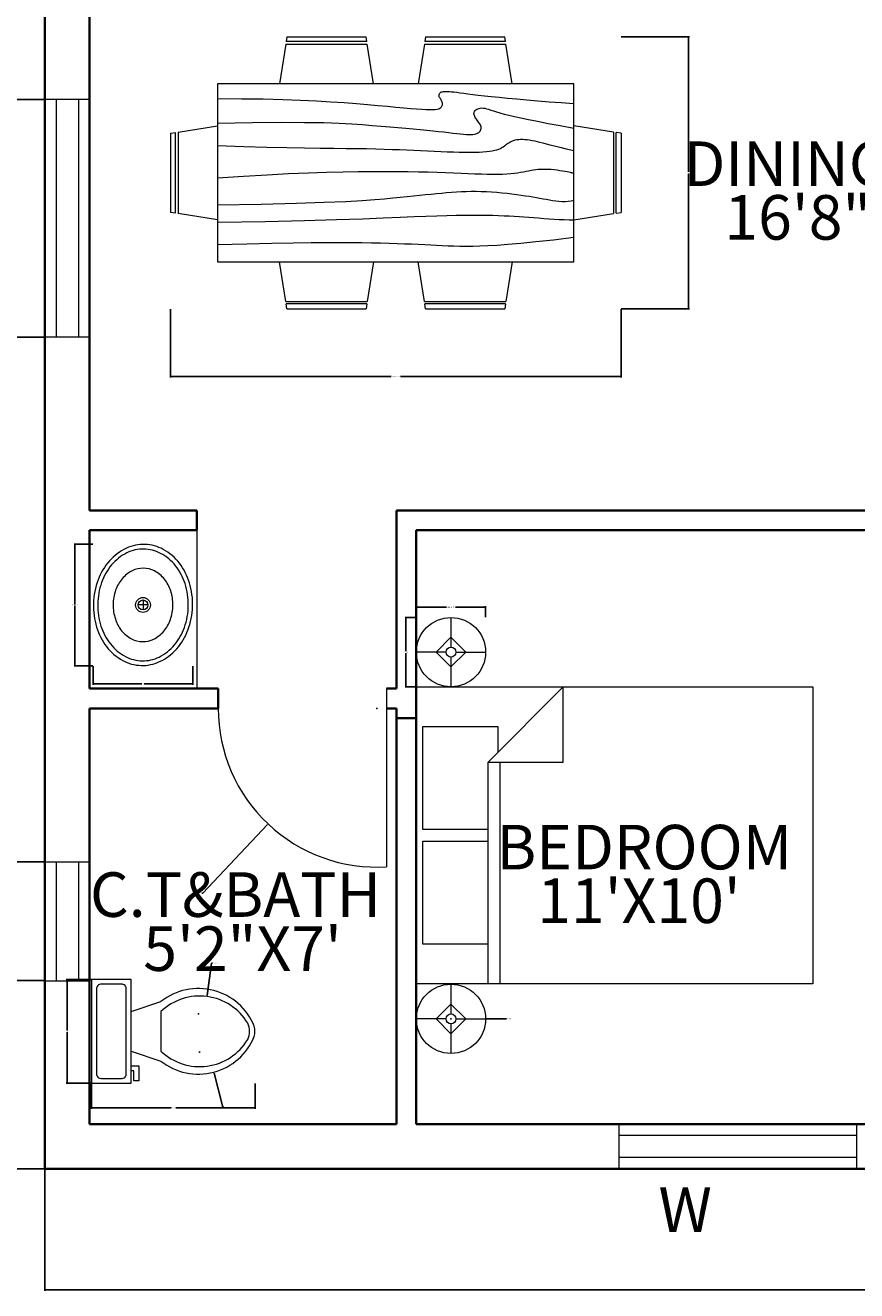
# Model space of a CAD drawing. Units: inches. Extents: x 2473 to 3664, y 1231 to 2079.
# Tile 3 of 8: x 2614 to 2782, y 1563 to 1819. Entities that reach past the tile are written whole.
import ezdxf

# ---------------------------------------------------------------- set-up
doc = ezdxf.new("R2010")
doc.units = ezdxf.units.IN
doc.linetypes.add('ACAD_ISO02W100', pattern=[15, 12, -3])
doc.layers.get('Defpoints').update_dxf_attribs({"linetype": 'ACAD_ISO02W100'})
for name, color, linetype, lineweight in [('A-ANNO-DIMS', 2, 'Continuous', 18), ('A-ANNO-IDEN', 7, 'Continuous', 18), ('A-AREA-IDEN', 7, 'Continuous', 18), ('A-DOOR', 4, 'Continuous', 18), ('A-FLOR-CASE', 9, 'Continuous', 18), ('A-FLOR-FIXT', 9, 'Continuous', 18), ('A-FURN', 8, 'Continuous', 13), ('A-GLAZ', 3, 'Continuous', 18), ('A-WALL', 7, 'Continuous', 35)]:
    doc.layers.add(name, color=color, linetype=linetype, lineweight=lineweight)
doc.styles.get("Standard").update_dxf_attribs({"font": 'arial.ttf'})
doc.dimstyles.get("Standard").update_dxf_attribs({"dimtxt": 0.18, "dimasz": 0.18, "dimexe": 0.18, "dimexo": 0.0625, "dimgap": 0.09, "dimtad": 0, "dimtih": 1, "dimtoh": 1, "dimdec": 4, "dimzin": 0, "dimdsep": 46, "dimtxsty": 'Standard', "dimcen": 0.09, "dimadec": 0, "dimazin": 0, "dimtfac": 1, "dimtdec": 4, "dimtofl": 0, "dimtmove": 0, "dimatfit": 3, "dimfxl": 1, "dimtolj": 1, "dimtzin": 0, "dimarcsym": 0})

# ---------------------------------------------------------------- blocks, each defined once
blk = doc.blocks.new('Bed - Queen')
for p, q in [((0, -80.00003), (0, 0)), ((0, 0), (59.99999, 0)), ((59.99999, 0), (59.99999, -80.00003)), ((7.99999, -1.2), (28.79998, -1.2)), ((7.99999, -14.4), (7.99999, -1.2)), ((28.79998, -1.2), (28.79998, -14.4)), ((31.19999, -1.2), (51.99999, -1.2)), ((31.19999, -14.4), (31.19999, -1.2)), ((51.99999, -1.2), (51.99999, -16.4)), ((0, -14.4), (44.8, -14.4)), ((59.99999, -29.6), (44.8, -14.4)), ((44.8, -14.4), (44.8, -29.6)), ((44.8, -16.8), (0, -16.8)), ((51.99999, -16.4), (46.79936, -16.4)), ((44.8, -29.6), (59.99999, -29.6)), ((59.99999, -80.00003), (0, -80.00003))]:
    blk.add_line(p, q)
blk = doc.blocks.new('Toilet - top')
for p, q in [((9.5, -6), (9.5, -2)), ((-10, -8.5), (-8, -8.5)), ((-10, -9.5), (-10, -8.5)), ((-7, -9.5), (-10, -9.5)), ((-8, -8.5), (-8, -8)), ((-7, -8), (-7, -9.5)), ((-4, -8), (-6, -14)), ((4, -8), (6, -14)), ((4, -14), (-4, -14))]:
    blk.add_line(p, q)
blk.add_lwpolyline([(10.5, -8), (10.5, 0), (-10.5, 0), (-10.5, -8)], close=True)
for points in [[(-9.5, -2), (-9.5, -6)], [(8.5, -1), (-8.5, -1)], [(-8.5, -7), (8.5, -7)]]:
    blk.add_lwpolyline(points)
for centre, radius, start, end in [((-8.62, -1.88), 0.884, 81.8699, 188.1301), ((8.62, -1.88), 0.884, 351.8699, 98.1301), ((-8.62, -6.12), 0.884, 171.8699, 278.1301), ((8.62, -6.12), 0.884, 261.8699, 8.1301), ((3.52, -21.58), 12.17, 141.4691, 247.9714), ((4.2, -21.82), 11.33, 136.3677, 238.9468), ((-3.52, -21.58), 12.17, 292.0284, 38.5307), ((-4.2, -21.82), 11.33, 301.053, 43.6321), ((0, -27.88), 4, 245.7318, 294.2682), ((0, -29), 4, 254.8605, 285.1395)]:
    blk.add_arc(centre, radius, start, end)
blk = doc.blocks.new('Dining Set - 36 x 72 in.')
for p, q in [((-22.2343, 26.00059), (-23.4847, 17.99762)), ((-22.2304, 26), (-5.7608, 26)), ((-22, 27.5), (-22.1562, 26.50042)), ((-5.8416, 26.5), (-22.1534, 26.5)), ((-22, 27.5), (-6, 27.5)), ((-5.8437, 26.49966), (-6, 27.5)), ((-4.5152, 17.99762), (-5.7655, 25.99926)), ((5.7657, 26.00059), (4.5153, 17.99762)), ((5.7696, 26), (22.2392, 26)), ((6, 27.5), (5.8438, 26.50042)), ((22.1584, 26.5), (5.8466, 26.5)), ((6, 27.5), (22, 27.5)), ((22.1563, 26.49966), (22, 27.5)), ((23.4848, 17.99762), (22.2345, 25.99926)), ((36, 18), (-36, 18)), ((-36, 18), (-36, -18)), ((36, -18), (36, 18)), ((-45.5, 8), (-44.5004, 8.15617)), ((-45.5, 8), (-45.5, -8)), ((-44.5, -8.15843), (-44.5, 8.15338)), ((-44.0006, 8.23428), (-35.9976, 9.48474)), ((-44, 8.23041), (-44, -8.23915)), ((44.0006, 8.23428), (35.9976, 9.48474)), ((44, 8.23041), (44, -8.23915)), ((44.5, -8.15843), (44.5, 8.15338)), ((45.5, 8), (44.5005, 8.15617)), ((45.5, 8), (45.5, -8)), ((-44.4997, -8.15631), (-45.5, -8)), ((-35.9976, -9.48476), (-43.9993, -8.2345)), ((35.9976, -9.48476), (43.9993, -8.2345)), ((44.4997, -8.15631), (45.5, -8)), ((-36, -18), (36, -18)), ((-22.2343, -26.0006), (-23.4847, -17.99762)), ((-4.5152, -17.99762), (-5.7655, -25.99928)), ((5.7657, -26.0006), (4.5153, -17.99762)), ((23.4848, -17.99762), (22.2345, -25.99928)), ((-22.2304, -26), (-5.7608, -26)), ((-22, -27.5), (-22.1562, -26.50044)), ((-5.8416, -26.5), (-22.1534, -26.5)), ((-22, -27.5), (-6, -27.5)), ((-5.8437, -26.49967), (-6, -27.5)), ((5.7696, -26), (22.2392, -26)), ((6, -27.5), (5.8438, -26.50044)), ((22.1584, -26.5), (5.8466, -26.5)), ((6, -27.5), (22, -27.5)), ((22.1563, -26.49967), (22, -27.5))]:
    blk.add_line(p, q)
for points in [[(-36, 15), (-31.1772, 14.97754), (-26.8079, 14.91406), (-22.8538, 14.81543), (-19.276, 14.6875), (-16.0362, 14.53613), (-13.0957, 14.36718), (-10.4159, 14.18652), (-7.9583, 14), (-5.6904, 13.81315), (-3.6035, 13.63021), (-1.6954, 13.45508), (0.0365, 13.29166), (1.5945, 13.14388), (2.9811, 13.01562), (4.1988, 12.9108), (5.25, 12.83333), (6.1393, 12.78613), (6.8802, 12.76823), (7.4883, 12.77767), (7.9792, 12.8125), (8.3685, 12.87077), (8.6719, 12.95052), (8.9049, 13.0498), (9.0833, 13.16666), (9.2205, 13.29899), (9.3216, 13.44401), (9.3895, 13.59879), (9.4271, 13.76041), (9.4373, 13.92594), (9.4232, 14.09245), (9.3875, 14.257), (9.3333, 14.41666), (9.2638, 14.56917), (9.1836, 14.71484), (9.0975, 14.85465), (9.0104, 14.98958), (8.9272, 15.1206), (8.8529, 15.2487), (8.7922, 15.37483), (8.75, 15.5), (8.7305, 15.62467), (8.7344, 15.74739), (8.7617, 15.86621), (8.8125, 15.97916), (8.8867, 16.08431), (8.9844, 16.17968), (9.1055, 16.26334), (9.25, 16.33333), (9.4189, 16.38802), (9.6172, 16.42708), (9.8506, 16.45052), (10.125, 16.45833), (10.4463, 16.45052), (10.8203, 16.42708), (11.2529, 16.38802), (11.75, 16.33333), (12.3184, 16.26318), (12.9694, 16.17838), (13.7151, 16.07991), (14.5677, 15.96875), (15.5395, 15.84586), (16.6426, 15.71224), (17.8893, 15.56884), (19.2917, 15.41666), (20.859, 15.25667), (22.5879, 15.08984), (24.4721, 14.91715), (26.5052, 14.73958), (28.6809, 14.5581), (30.9929, 14.3737), (33.4347, 14.18733), (36, 14)], [(-36, 10), (-28.9766, 10.14274), (-23.1725, 10.20442), (-18.4241, 10.19775), (-14.5677, 10.13541), (-11.4399, 10.03011), (-8.877, 9.89453), (-6.7154, 9.74137), (-4.7917, 9.58333), (-2.9698, 9.43082), (-1.2246, 9.28515), (0.4415, 9.14534), (2.026, 9.01041), (3.5266, 8.87939), (4.9408, 8.7513), (6.266, 8.62516), (7.5, 8.5), (8.6411, 8.37549), (9.6914, 8.2539), (10.6538, 8.13818), (11.5312, 8.03125), (12.3267, 7.93603), (13.043, 7.85547), (13.6831, 7.79248), (14.25, 7.75), (14.7471, 7.7303), (15.1797, 7.73307), (15.5537, 7.75732), (15.875, 7.80208), (16.1494, 7.86637), (16.3828, 7.94922), (16.5811, 8.04964), (16.75, 8.16666), (16.8944, 8.29915), (17.0143, 8.44531), (17.1089, 8.60319), (17.1771, 8.77083), (17.218, 8.94629), (17.2305, 9.1276), (17.2137, 9.31282), (17.1667, 9.5), (17.0895, 9.6875), (16.987, 9.875), (16.8649, 10.0625), (16.7292, 10.25), (16.5856, 10.4375), (16.4401, 10.625), (16.2985, 10.8125), (16.1667, 11), (16.05, 11.18733), (15.9518, 11.3737), (15.8752, 11.5581), (15.8229, 11.73958), (15.798, 11.91715), (15.8034, 12.08984), (15.842, 12.25667), (15.9167, 12.41666), (16.0295, 12.56836), (16.1784, 12.70833), (16.3605, 12.83268), (16.5729, 12.9375), (16.8127, 13.01888), (17.0768, 13.07291), (17.3625, 13.0957), (17.6667, 13.08333), (17.9894, 13.03312), (18.3418, 12.94726), (18.7382, 12.82918), (19.1927, 12.68229), (19.7195, 12.51001), (20.3327, 12.31575), (21.0465, 12.10294), (21.875, 11.875), (22.8357, 11.63354), (23.959, 11.37304), (25.2786, 11.08618), (26.8282, 10.76562), (28.6414, 10.40405), (30.752, 9.99414), (33.1936, 9.52856), (36, 9)], [(-36, 5.5), (-30.7157, 5.3348), (-26.069, 5.20963), (-21.9946, 5.11767), (-18.4271, 5.05208), (-15.3009, 5.00602), (-12.5508, 4.97265), (-10.1112, 4.94515), (-7.9167, 4.91666), (-5.909, 4.88167), (-4.0586, 4.83984), (-2.3429, 4.79215), (-0.7396, 4.73958), (0.7739, 4.6831), (2.22, 4.6237), (3.6213, 4.56233), (5, 4.5), (6.373, 4.43782), (7.7344, 4.3776), (9.0723, 4.32129), (10.375, 4.27083), (11.6309, 4.22819), (12.8281, 4.19531), (13.9551, 4.17415), (15, 4.16666), (15.954, 4.17448), (16.819, 4.19791), (17.6001, 4.23698), (18.3021, 4.29166), (18.9299, 4.36198), (19.4883, 4.44791), (19.9823, 4.54948), (20.4167, 4.66666), (20.7969, 4.79899), (21.1302, 4.94401), (21.4245, 5.09879), (21.6875, 5.26041), (21.9271, 5.42594), (22.1511, 5.59245), (22.3672, 5.757), (22.5834, 5.91666), (22.8065, 6.06868), (23.0404, 6.21093), (23.2879, 6.34147), (23.5521, 6.45833), (23.8358, 6.55957), (24.142, 6.64323), (24.4735, 6.70735), (24.8334, 6.75), (25.2235, 6.76969), (25.642, 6.76692), (26.0858, 6.74267), (26.5521, 6.69791), (27.0379, 6.63362), (27.5404, 6.55078), (28.0565, 6.45036), (28.5834, 6.33333), (29.1242, 6.19987), (29.7071, 6.04687), (30.3661, 5.87044), (31.1354, 5.66666), (32.0493, 5.43164), (33.142, 5.16146), (34.4475, 4.85221), (36, 4.5)], [(-36, -1), (-30.7915, -0.6591), (-26.0195, -0.38216), (-21.6519, -0.16284), (-17.6563, 0.00521), (-14.0005, 0.12833), (-10.6523, 0.21289), (-7.5796, 0.26522), (-4.75, 0.29166), (-2.134, 0.29793), (0.2878, 0.28711), (2.5317, 0.26163), (4.6146, 0.22396), (6.5529, 0.17651), (8.3633, 0.12174), (10.0623, 0.06209), (11.6667, 0), (13.1899, -0.06201), (14.6341, -0.1211), (15.9982, -0.17432), (17.2813, -0.21875), (18.4823, -0.25147), (19.6003, -0.26953), (20.6343, -0.27002), (21.5834, -0.25), (22.4481, -0.20768), (23.2357, -0.14584), (23.9549, -0.06836), (24.6146, 0.02083), (25.2235, 0.11784), (25.7904, 0.21875), (26.3241, 0.31966), (26.8334, 0.41666), (27.3265, 0.50618), (27.8099, 0.58593), (28.2894, 0.65397), (28.7709, 0.70833), (29.2601, 0.74707), (29.763, 0.76823), (30.2855, 0.76985), (30.8334, 0.75), (31.4088, 0.70784), (31.9994, 0.64713), (32.589, 0.57275), (33.1615, 0.48958), (33.7008, 0.4025), (34.1908, 0.3164), (34.6153, 0.23616), (34.9584, 0.16666), (35.2099, 0.11165), (35.3848, 0.07031), (35.504, 0.04069), (35.5886, 0.02083), (35.6594, 0.00879), (35.7377, 0.0026), (35.8442, 0.00032), (36, 0)], [(-36, -6.5), (-27.1843, -6.31267), (-20.084, -6.1263), (-14.469, -5.9419), (-10.1094, -5.76042), (-6.7752, -5.58285), (-4.2363, -5.41016), (-2.2629, -5.24333), (-0.625, -5.08334), (0.8708, -4.93099), (2.2715, -4.78646), (3.5872, -4.64974), (4.8281, -4.52084), (6.0046, -4.39974), (7.127, -4.28646), (8.2053, -4.18099), (9.25, -4.08334), (10.2705, -3.99382), (11.2734, -3.91407), (12.2647, -3.84603), (13.25, -3.79167), (14.2354, -3.75293), (15.2266, -3.73177), (16.2295, -3.73015), (17.25, -3.75), (18.2912, -3.79248), (19.3451, -3.85547), (20.4009, -3.93604), (21.4479, -4.03125), (22.4754, -4.13819), (23.4727, -4.25391), (24.4289, -4.37549), (25.3334, -4.5), (26.1785, -4.62492), (26.9694, -4.74935), (27.7145, -4.87281), (28.4219, -4.99479), (29.1, -5.11483), (29.7572, -5.23242), (30.4016, -5.34709), (31.0417, -5.45834), (31.6837, -5.56437), (32.3262, -5.65821), (32.9658, -5.73153), (33.599, -5.77604), (34.2224, -5.78345), (34.8327, -5.74545), (35.4264, -5.65373), (36, -5.5)], [(-36, -10), (-26.4022, -9.81299), (-18.4675, -9.62891), (-11.9839, -9.45069), (-6.7396, -9.28125), (-2.5226, -9.12354), (0.8789, -8.98047), (3.6769, -8.85498), (6.0833, -8.75), (8.2767, -8.66765), (10.3021, -8.60677), (12.1712, -8.56543), (13.8958, -8.54167), (15.4876, -8.53353), (16.9583, -8.53907), (18.3197, -8.55632), (19.5834, -8.58334), (20.7616, -8.61841), (21.8685, -8.66081), (22.9188, -8.71004), (23.9271, -8.76563), (24.9081, -8.82707), (25.8763, -8.89388), (26.8465, -8.96558), (27.8334, -9.04167), (28.8474, -9.12118), (29.8828, -9.20117), (30.93, -9.27824), (31.9792, -9.34896), (33.0205, -9.40991), (34.0443, -9.45768), (35.0407, -9.48885), (36, -9.5)], [(-36, -14.5), (-30.0881, -14.33513), (-25.0332, -14.21224), (-20.7312, -14.12647), (-17.0781, -14.07292), (-13.97, -14.04671), (-11.3027, -14.04297), (-8.9724, -14.05681), (-6.875, -14.08334), (-4.9224, -14.11833), (-3.0905, -14.16016), (-1.3709, -14.20785), (0.2448, -14.26042), (1.7647, -14.3169), (3.1973, -14.3763), (4.5507, -14.43767), (5.8333, -14.5), (7.0554, -14.5621), (8.235, -14.62175), (9.3922, -14.67652), (10.5469, -14.72396), (11.7192, -14.76164), (12.929, -14.78711), (14.1965, -14.79794), (15.5417, -14.79167), (16.9933, -14.76424), (18.6152, -14.70508), (20.4804, -14.60197), (22.6615, -14.44271), (25.2312, -14.21509), (28.2624, -13.9069), (31.8277, -13.50594), (36, -13)]]:
    blk.add_lwpolyline(points)
blk = doc.blocks.new('Lamp - Table')
for p, q in [((0, 7), (0, 1)), ((0, 3), (-3, 0)), ((3, 0), (0, 3)), ((-1, 0), (-7, 0)), ((-3, 0), (0, -3)), ((0, -3), (3, 0)), ((1, 0), (7, 0)), ((0, -1), (0, -7))]:
    blk.add_line(p, q)
for radius in [7, 1]:
    blk.add_circle((0, 0), radius)
blk = doc.blocks.new('Sink - Oval top')
for p, q in [((-1, 0), (1, 0)), ((0, 1), (0, -1))]:
    blk.add_line(p, q)
for points in [[(-12.23, 0.39, 0.117634), (-11.46, -3.36, 0.104469), (-8.88, -6.8, 0.090016), (-5.08, -9.07, 0.08192), (-0.32, -10.02, 0.08192), (4.49, -9.38, 0.090016), (8.42, -7.36, 0.104469), (11.22, -4.09, 0.117634), (12.23, -0.39, 0.117634), (11.46, 3.36, 0.104469), (8.88, 6.8, 0.090016), (5.08, 9.07, 0.08192), (0.32, 10.02, 0.08192), (-4.49, 9.38, 0.090016), (-8.42, 7.36, 0.104469), (-11.22, 4.09, 0.117634)], [(-11.29, 0.16, 0.118622), (-10.52, -3.25, 0.104678), (-8.07, -6.36, 0.089562), (-4.54, -8.37, 0.081185), (-0.13, -9.15, 0.081185), (4.3, -8.49, 0.089562), (7.89, -6.58, 0.104678), (10.42, -3.55, 0.118622), (11.29, -0.16, 0.118622), (10.52, 3.25, 0.104678), (8.07, 6.36, 0.089562), (4.54, 8.37, 0.081185), (0.13, 9.15, 0.081185), (-4.3, 8.49, 0.089562), (-7.89, 6.58, 0.104678), (-10.42, 3.55, 0.118622)], [(-7.42, 0.08, 0.118283), (-6.91, -2.17, 0.104607), (-5.29, -4.21, 0.089718), (-2.97, -5.53, 0.081436), (-0.07, -6.04, 0.081436), (2.84, -5.59, 0.089718), (5.2, -4.33, 0.104607), (6.86, -2.32, 0.118283), (7.42, -0.08, 0.118283), (6.91, 2.17, 0.104607), (5.29, 4.21, 0.089718), (2.97, 5.53, 0.081436), (0.07, 6.04, 0.081436), (-2.84, 5.59, 0.089718), (-5.2, 4.33, 0.104607), (-6.86, 2.32, 0.118283)]]:
    blk.add_lwpolyline(points, format="xyb", close=True)
for radius in [1.5, 1]:
    blk.add_circle((0, 0), radius)
blk = doc.blocks.new('GLAZ-PLAN-48')
for p, q in [((0, 9), (0, 0)), ((48, 9), (48, 0)), ((0, 6.75), (48, 6.75)), ((0, 2.25), (48, 2.25))]:
    blk.add_line(p, q)
blk = doc.blocks.new('*D19')
at = {"layer": 'A-ANNO-DIMS', "color": 0, "lineweight": -2, "transparency": 16777216}
for p, q in [((2692.7, 1699.49), (2692.7, 1701.7)), ((2692.88, 1701.52), (2698.8, 1701.52)), ((2706.52, 1701.52), (2700.6, 1701.52)), ((2706.7, 1699.49), (2706.7, 1701.7))]:
    blk.add_line(p, q, dxfattribs=at)
at = {"layer": 'A-ANNO-DIMS', "color": 0, "transparency": 16777216}
for points in [[(2692.88, 1701.55), (2692.88, 1701.49), (2692.7, 1701.52)], [(2706.52, 1701.55), (2706.52, 1701.49), (2706.7, 1701.52)]]:
    blk.add_solid(points, dxfattribs=at)
at = {"layer": 'Defpoints', "color": 0, "transparency": 16777216}
for p in [(2706.7, 1701.52), (2692.7, 1699.42), (2706.7, 1699.42)]:
    blk.add_point(p, dxfattribs=at)
at = {"layer": 'A-ANNO-DIMS', "color": 0, "transparency": 16777216, "insert": (2699.7, 1701.52), "char_height": 0.18, "attachment_point": 5}
blk.add_mtext('\\A1;LAMP 14 TYP.', dxfattribs=at)
blk = doc.blocks.new('*D20')
at = {"layer": 'A-ANNO-DIMS', "color": 0, "lineweight": -2, "transparency": 16777216}
for p, q in [((2692.63, 1699.42), (2690.42, 1699.42)), ((2690.6, 1699.24), (2690.6, 1692.61)), ((2690.6, 1685.6), (2690.6, 1692.24)), ((2692.63, 1685.42), (2690.42, 1685.42))]:
    blk.add_line(p, q, dxfattribs=at)
at = {"layer": 'A-ANNO-DIMS', "color": 0, "transparency": 16777216}
for points in [[(2690.57, 1699.24), (2690.63, 1699.24), (2690.6, 1699.42)], [(2690.57, 1685.6), (2690.63, 1685.6), (2690.6, 1685.42)]]:
    blk.add_solid(points, dxfattribs=at)
at = {"layer": 'Defpoints', "color": 0, "transparency": 16777216}
for p in [(2690.6, 1699.42), (2692.7, 1699.42), (2692.7, 1685.42)]:
    blk.add_point(p, dxfattribs=at)
at = {"layer": 'A-ANNO-DIMS', "color": 0, "transparency": 16777216, "insert": (2690.6, 1692.42), "char_height": 0.18, "attachment_point": 5}
blk.add_mtext('\\A1;14 TYP.', dxfattribs=at)
blk = doc.blocks.new('*D39')
at = {"layer": 'A-ANNO-DIMS', "color": 0, "lineweight": -2, "transparency": 16777216}
for p, q in [((2627.1, 1605.26), (2627.1, 1600.19)), ((2660.14, 1605.26), (2660.14, 1600.19)), ((2627.28, 1600.37), (2643.15, 1600.37)), ((2659.96, 1600.37), (2644.09, 1600.37))]:
    blk.add_line(p, q, dxfattribs=at)
at = {"layer": 'A-ANNO-DIMS', "color": 0, "transparency": 16777216}
for points in [[(2627.28, 1600.4), (2627.28, 1600.34), (2627.1, 1600.37)], [(2659.96, 1600.4), (2659.96, 1600.34), (2660.14, 1600.37)]]:
    blk.add_solid(points, dxfattribs=at)
at = {"layer": 'Defpoints', "color": 0, "transparency": 16777216}
for p in [(2627.1, 1605.32), (2660.14, 1605.32), (2627.1, 1600.37)]:
    blk.add_point(p, dxfattribs=at)
at = {"layer": 'A-ANNO-DIMS', "color": 0, "transparency": 16777216, "insert": (2643.62, 1600.37), "char_height": 0.18, "attachment_point": 5}
blk.add_mtext('\\A1;WC 33', dxfattribs=at)
blk = doc.blocks.new('*D40')
at = {"layer": 'A-ANNO-DIMS', "color": 0, "lineweight": -2, "transparency": 16777216}
for p, q in [((2627.04, 1626.32), (2621.96, 1626.32)), ((2622.14, 1626.14), (2622.14, 1616.01)), ((2622.14, 1605.5), (2622.14, 1615.64)), ((2627.04, 1605.32), (2621.96, 1605.32))]:
    blk.add_line(p, q, dxfattribs=at)
at = {"layer": 'A-ANNO-DIMS', "color": 0, "transparency": 16777216}
for points in [[(2622.11, 1626.14), (2622.17, 1626.14), (2622.14, 1626.32)], [(2622.11, 1605.5), (2622.17, 1605.5), (2622.14, 1605.32)]]:
    blk.add_solid(points, dxfattribs=at)
at = {"layer": 'Defpoints', "color": 0, "transparency": 16777216}
for p in [(2622.14, 1626.32), (2627.1, 1626.32), (2627.1, 1605.32)]:
    blk.add_point(p, dxfattribs=at)
at = {"layer": 'A-ANNO-DIMS', "color": 0, "transparency": 16777216, "insert": (2622.14, 1615.82), "char_height": 0.18, "attachment_point": 5}
blk.add_mtext('\\A1;21', dxfattribs=at)
blk = doc.blocks.new('*D41')
at = {"layer": 'A-ANNO-DIMS', "color": 0, "lineweight": -2, "transparency": 16777216}
for p, q in [((2643.05, 1761.69), (2643.05, 1747.93)), ((2734.05, 1761.69), (2734.05, 1747.93)), ((2643.23, 1748.11), (2687.6, 1748.11)), ((2733.87, 1748.11), (2689.5, 1748.11))]:
    blk.add_line(p, q, dxfattribs=at)
at = {"layer": 'A-ANNO-DIMS', "color": 0, "transparency": 16777216}
for points in [[(2643.23, 1748.14), (2643.23, 1748.08), (2643.05, 1748.11)], [(2733.87, 1748.14), (2733.87, 1748.08), (2734.05, 1748.11)]]:
    blk.add_solid(points, dxfattribs=at)
at = {"layer": 'Defpoints', "color": 0, "transparency": 16777216}
for p in [(2643.05, 1761.76), (2734.05, 1761.76), (2734.05, 1748.11)]:
    blk.add_point(p, dxfattribs=at)
at = {"layer": 'A-ANNO-DIMS', "color": 0, "transparency": 16777216, "insert": (2688.55, 1748.11), "char_height": 0.18, "attachment_point": 5}
blk.add_mtext('\\A1;DINING SET 91', dxfattribs=at)
blk = doc.blocks.new('*D42')
at = {"layer": 'A-ANNO-DIMS', "color": 0, "lineweight": -2, "transparency": 16777216}
for p, q in [((2734.11, 1816.76), (2747.88, 1816.76)), ((2747.7, 1816.58), (2747.7, 1789.44)), ((2747.7, 1761.94), (2747.7, 1789.07)), ((2734.11, 1761.76), (2747.88, 1761.76))]:
    blk.add_line(p, q, dxfattribs=at)
at = {"layer": 'A-ANNO-DIMS', "color": 0, "transparency": 16777216}
for points in [[(2747.67, 1816.58), (2747.73, 1816.58), (2747.7, 1816.76)], [(2747.67, 1761.94), (2747.73, 1761.94), (2747.7, 1761.76)]]:
    blk.add_solid(points, dxfattribs=at)
at = {"layer": 'Defpoints', "color": 0, "transparency": 16777216}
for p in [(2734.05, 1816.76), (2747.7, 1816.76), (2734.05, 1761.76)]:
    blk.add_point(p, dxfattribs=at)
at = {"layer": 'A-ANNO-DIMS', "color": 0, "transparency": 16777216, "insert": (2747.7, 1789.26), "char_height": 0.18, "attachment_point": 5}
blk.add_mtext('\\A1;55', dxfattribs=at)
blk = doc.blocks.new('*D43')
at = {"layer": 'A-ANNO-DIMS', "color": 0, "lineweight": -2, "transparency": 16777216}
for p, q in [((2627.35, 1714.24), (2623.54, 1714.24)), ((2623.72, 1714.06), (2623.72, 1702.14)), ((2623.72, 1689.87), (2623.72, 1701.78)), ((2627.35, 1689.69), (2623.54, 1689.69))]:
    blk.add_line(p, q, dxfattribs=at)
at = {"layer": 'A-ANNO-DIMS', "color": 0, "transparency": 16777216}
for points in [[(2623.69, 1714.06), (2623.75, 1714.06), (2623.72, 1714.24)], [(2623.69, 1689.87), (2623.75, 1689.87), (2623.72, 1689.69)]]:
    blk.add_solid(points, dxfattribs=at)
at = {"layer": 'Defpoints', "color": 0, "transparency": 16777216}
for p in [(2627.41, 1714.24), (2623.72, 1689.69), (2627.41, 1689.69)]:
    blk.add_point(p, dxfattribs=at)
at = {"layer": 'A-ANNO-DIMS', "color": 0, "transparency": 16777216, "insert": (2623.72, 1701.96), "char_height": 0.18, "attachment_point": 5}
blk.add_mtext('\\A1;BASIN 25', dxfattribs=at)
blk = doc.blocks.new('*D44')
at = {"layer": 'A-ANNO-DIMS', "color": 0, "lineweight": -2, "transparency": 16777216}
for p, q in [((2627.41, 1689.62), (2627.41, 1685.82)), ((2647.54, 1689.62), (2647.54, 1685.82)), ((2627.59, 1686), (2637.26, 1686)), ((2647.36, 1686), (2637.7, 1686))]:
    blk.add_line(p, q, dxfattribs=at)
at = {"layer": 'A-ANNO-DIMS', "color": 0, "transparency": 16777216}
for points in [[(2627.59, 1686.03), (2627.59, 1685.97), (2627.41, 1686)], [(2647.36, 1686.03), (2647.36, 1685.97), (2647.54, 1686)]]:
    blk.add_solid(points, dxfattribs=at)
at = {"layer": 'Defpoints', "color": 0, "transparency": 16777216}
for p in [(2627.41, 1689.69), (2647.54, 1689.69), (2647.54, 1686)]:
    blk.add_point(p, dxfattribs=at)
at = {"layer": 'A-ANNO-DIMS', "color": 0, "transparency": 16777216, "insert": (2637.48, 1686), "char_height": 0.18, "attachment_point": 5}
blk.add_mtext('\\A1;20', dxfattribs=at)
blk = doc.blocks.new('*D49')
at = {"layer": 'A-ANNO-DIMS', "color": 0, "lineweight": -2, "transparency": 16777216}
for p, q in [((2995.66, 1644.99), (2995.66, 1563.43)), ((2617.66, 1587.99), (2617.66, 1563.43)), ((2617.84, 1563.61), (2806.37, 1563.61)), ((2995.48, 1563.61), (2806.95, 1563.61))]:
    blk.add_line(p, q, dxfattribs=at)
at = {"layer": 'A-ANNO-DIMS', "color": 0, "transparency": 16777216}
for points in [[(2617.84, 1563.64), (2617.84, 1563.58), (2617.66, 1563.61)], [(2995.48, 1563.64), (2995.48, 1563.58), (2995.66, 1563.61)]]:
    blk.add_solid(points, dxfattribs=at)
at = {"layer": 'Defpoints', "color": 0, "transparency": 16777216}
for p in [(2995.66, 1645.06), (2617.66, 1588.06), (2995.66, 1563.61)]:
    blk.add_point(p, dxfattribs=at)
at = {"layer": 'A-ANNO-DIMS', "color": 0, "transparency": 16777216, "insert": (2806.66, 1563.61), "char_height": 0.18, "attachment_point": 5}
blk.add_mtext('\\A1;378', dxfattribs=at)
blk = doc.blocks.new('*D50')
at = {"layer": 'A-ANNO-DIMS', "color": 0, "lineweight": -2, "transparency": 16777216}
for p, q in [((2746.72, 2006.06), (3020.29, 2006.06)), ((3020.11, 2005.88), (3020.11, 1797.24)), ((3020.11, 1588.24), (3020.11, 1796.87)), ((2844.72, 1588.06), (3020.29, 1588.06))]:
    blk.add_line(p, q, dxfattribs=at)
at = {"layer": 'A-ANNO-DIMS', "color": 0, "transparency": 16777216}
for points in [[(3020.08, 2005.88), (3020.14, 2005.88), (3020.11, 2006.06)], [(3020.08, 1588.24), (3020.14, 1588.24), (3020.11, 1588.06)]]:
    blk.add_solid(points, dxfattribs=at)
at = {"layer": 'Defpoints', "color": 0, "transparency": 16777216}
for p in [(2746.66, 2006.06), (3020.11, 2006.06), (2844.66, 1588.06)]:
    blk.add_point(p, dxfattribs=at)
at = {"layer": 'A-ANNO-DIMS', "color": 0, "transparency": 16777216, "insert": (3020.11, 1797.06), "char_height": 0.18, "attachment_point": 5}
blk.add_mtext('\\A1;418', dxfattribs=at)
blk = doc.blocks.new('*D57')
at = {"layer": 'A-ANNO-DIMS', "color": 0, "lineweight": -2, "transparency": 16777216}
for p, q in [((2617.6, 1626.06), (2593.03, 1626.06)), ((2593.21, 1625.88), (2593.21, 1607.24)), ((2593.21, 1588.24), (2593.21, 1606.87)), ((2617.6, 1588.06), (2593.03, 1588.06))]:
    blk.add_line(p, q, dxfattribs=at)
at = {"layer": 'A-ANNO-DIMS', "color": 0, "transparency": 16777216}
for points in [[(2593.18, 1625.88), (2593.24, 1625.88), (2593.21, 1626.06)], [(2593.18, 1588.24), (2593.24, 1588.24), (2593.21, 1588.06)]]:
    blk.add_solid(points, dxfattribs=at)
at = {"layer": 'Defpoints', "color": 0, "transparency": 16777216}
for p in [(2593.21, 1626.06), (2617.66, 1626.06), (2617.66, 1588.06)]:
    blk.add_point(p, dxfattribs=at)
at = {"layer": 'A-ANNO-DIMS', "color": 0, "transparency": 16777216, "insert": (2593.21, 1607.06), "char_height": 0.18, "attachment_point": 5}
blk.add_mtext('\\A1;38', dxfattribs=at)
blk = doc.blocks.new('*D58')
at = {"layer": 'A-ANNO-DIMS', "color": 0, "lineweight": -2, "transparency": 16777216}
for p, q in [((2617.6, 1756.06), (2593.03, 1756.06)), ((2593.21, 1755.88), (2593.21, 1703.24)), ((2593.21, 1650.24), (2593.21, 1702.87)), ((2617.6, 1650.06), (2593.03, 1650.06))]:
    blk.add_line(p, q, dxfattribs=at)
at = {"layer": 'A-ANNO-DIMS', "color": 0, "transparency": 16777216}
for points in [[(2593.18, 1755.88), (2593.24, 1755.88), (2593.21, 1756.06)], [(2593.18, 1650.24), (2593.24, 1650.24), (2593.21, 1650.06)]]:
    blk.add_solid(points, dxfattribs=at)
at = {"layer": 'Defpoints', "color": 0, "transparency": 16777216}
for p in [(2593.21, 1756.06), (2617.66, 1756.06), (2617.66, 1650.06)]:
    blk.add_point(p, dxfattribs=at)
at = {"layer": 'A-ANNO-DIMS', "color": 0, "transparency": 16777216, "insert": (2593.21, 1703.06), "char_height": 0.18, "attachment_point": 5}
blk.add_mtext('\\A1;106', dxfattribs=at)
blk = doc.blocks.new('*D59')
at = {"layer": 'A-ANNO-DIMS', "color": 0, "lineweight": -2, "transparency": 16777216}
for p, q in [((2617.597908, 1881.056109), (2593.030408, 1881.056109)), ((2593.210408, 1880.876109), (2593.210408, 1842.736109)), ((2593.210408, 1804.236109), (2593.210408, 1842.376109)), ((2617.597908, 1804.056109), (2593.030408, 1804.056109))]:
    blk.add_line(p, q, dxfattribs=at)
at = {"layer": 'A-ANNO-DIMS', "color": 0, "transparency": 16777216}
for points in [[(2593.180408, 1880.876109), (2593.240408, 1880.876109), (2593.210408, 1881.056109)], [(2593.180408, 1804.236109), (2593.240408, 1804.236109), (2593.210408, 1804.056109)]]:
    blk.add_solid(points, dxfattribs=at)
at = {"layer": 'Defpoints', "color": 0, "transparency": 16777216}
for p in [(2593.210408, 1881.056109), (2617.660408, 1881.056109), (2617.660408, 1804.056109)]:
    blk.add_point(p, dxfattribs=at)
at = {"layer": 'A-ANNO-DIMS', "color": 0, "transparency": 16777216, "insert": (2593.210408, 1842.556109), "char_height": 0.18, "attachment_point": 5}
blk.add_mtext('\\A1;77', dxfattribs=at)
blk = doc.blocks.new('*D110')
at = {"layer": 'A-ANNO-DIMS', "color": 0, "lineweight": -2, "transparency": 16777216}
for p, q in [((2684.63, 1681.06), (2684.81, 1681.06)), ((2684.72, 1680.97), (2684.72, 1681.15)), ((2649.56, 1643.7), (2662.62, 1657.58)), ((2649.38, 1643.7), (2649.56, 1643.7))]:
    blk.add_line(p, q, dxfattribs=at)
at = {"layer": 'A-ANNO-DIMS', "color": 0, "transparency": 16777216}
blk.add_solid([(2662.6, 1657.6), (2662.65, 1657.56), (2662.75, 1657.71)], dxfattribs=at)
at = {"layer": 'Defpoints', "color": 0, "transparency": 16777216}
for p in [(2684.72, 1681.06), (2662.75, 1657.71)]:
    blk.add_point(p, dxfattribs=at)
at = {"layer": 'A-ANNO-DIMS', "color": 0, "transparency": 16777216, "insert": (2648.9, 1643.7), "char_height": 0.18, "attachment_point": 5}
blk.add_mtext('\\A1;R32.06', dxfattribs=at)
blk = doc.blocks.new('*D112')
at = {"layer": 'A-ANNO-DIMS', "color": 0, "lineweight": -2, "transparency": 16777216}
for p, q in [((2648.59, 1619.34), (2648.77, 1619.34)), ((2648.68, 1619.25), (2648.68, 1619.43)), ((2653.63, 1600.51), (2651.82, 1607.4)), ((2653.81, 1600.51), (2653.63, 1600.51))]:
    blk.add_line(p, q, dxfattribs=at)
at = {"layer": 'A-ANNO-DIMS', "color": 0, "transparency": 16777216}
blk.add_solid([(2651.85, 1607.41), (2651.79, 1607.39), (2651.77, 1607.57)], dxfattribs=at)
at = {"layer": 'Defpoints', "color": 0, "transparency": 16777216}
for p in [(2648.68, 1619.34), (2651.77, 1607.57)]:
    blk.add_point(p, dxfattribs=at)
at = {"layer": 'A-ANNO-DIMS', "color": 0, "transparency": 16777216, "insert": (2654.48, 1600.51), "char_height": 0.18, "attachment_point": 5}
blk.add_mtext('\\A1;2X R12.17', dxfattribs=at)
blk = doc.blocks.new('*D113')
at = {"layer": 'A-ANNO-DIMS', "color": 0, "lineweight": -2, "transparency": 16777216}
for p, q in [((2651.33, 1629.59), (2650.45, 1623.03)), ((2651.51, 1629.59), (2651.33, 1629.59)), ((2648.83, 1611.63), (2649.01, 1611.63)), ((2648.92, 1611.54), (2648.92, 1611.72))]:
    blk.add_line(p, q, dxfattribs=at)
at = {"layer": 'A-ANNO-DIMS', "color": 0, "transparency": 16777216}
blk.add_solid([(2650.42, 1623.04), (2650.48, 1623.03), (2650.43, 1622.85)], dxfattribs=at)
at = {"layer": 'Defpoints', "color": 0, "transparency": 16777216}
for p in [(2650.43, 1622.85), (2648.92, 1611.63)]:
    blk.add_point(p, dxfattribs=at)
at = {"layer": 'A-ANNO-DIMS', "color": 0, "transparency": 16777216, "insert": (2652.19, 1629.59), "char_height": 0.18, "attachment_point": 5}
blk.add_mtext('\\A1;2X R11.33', dxfattribs=at)
blk = doc.blocks.new('*D114')
at = {"layer": 'A-ANNO-DIMS', "color": 0, "lineweight": -2, "transparency": 16777216}
for p, q in [((2699.6, 1618.34), (2699.78, 1618.34)), ((2699.69, 1618.25), (2699.69, 1618.43)), ((2710.89, 1618.34), (2706.87, 1618.34))]:
    blk.add_line(p, q, dxfattribs=at)
at = {"layer": 'A-ANNO-DIMS', "color": 0, "transparency": 16777216}
blk.add_solid([(2706.87, 1618.37), (2706.87, 1618.31), (2706.69, 1618.34)], dxfattribs=at)
at = {"layer": 'Defpoints', "color": 0, "transparency": 16777216}
for p in [(2692.69, 1618.34), (2706.69, 1618.34)]:
    blk.add_point(p, dxfattribs=at)
at = {"layer": 'A-ANNO-DIMS', "color": 0, "transparency": 16777216, "insert": (2711.4, 1618.34), "char_height": 0.18, "attachment_point": 5}
blk.add_mtext('\\A1;4X ∅14', dxfattribs=at)

msp = doc.modelspace()

# ---------------------------------------------------------------- linework, layer by layer
at = {"layer": 'A-DOOR'}
msp.add_line((2686.6604, 1685.0561), (2686.6604, 1649.0561), dxfattribs=at)
msp.add_arc((2684.7192, 1681.0561), 32.0588, 180, 273.471409, dxfattribs=at)
at = {"layer": 'A-FLOR-CASE'}
msp.add_line((2648.3272, 1717.0561), (2648.3272, 1685.0561), dxfattribs=at)
at = {"layer": 'A-GLAZ'}
for p, q in [((2617.6604, 1650.0561), (2626.6604, 1650.0561)), ((2619.9104, 1650.0561), (2619.9104, 1626.0561)), ((2624.4104, 1650.0561), (2624.4104, 1626.0561)), ((2617.6604, 1626.0561), (2626.6604, 1626.0561))]:
    msp.add_line(p, q, dxfattribs=at)
at = {"layer": 'A-WALL'}
for p, q in [((2617.6604, 1970.0561), (2617.6604, 1588.0561)), ((2626.6604, 1837.0561), (2626.6604, 1721.0561)), ((2626.6604, 1721.0561), (2648.3272, 1721.0561)), ((2648.3272, 1721.0561), (2648.3272, 1717.0561)), ((2688.6604, 1721.0561), (2688.6604, 1717.0561)), ((2688.6604, 1721.0561), (2800.6604, 1721.0561)), ((2688.6604, 1721.0561), (2688.6604, 1685.0561)), ((2626.6604, 1717.0561), (2648.3272, 1717.0561)), ((2626.6604, 1717.0561), (2626.6604, 1685.0561)), ((2692.6604, 1717.0561), (2692.6604, 1597.0561)), ((2692.6604, 1717.0561), (2800.6604, 1717.0561)), ((2626.6604, 1685.0561), (2652.6604, 1685.0561)), ((2652.6604, 1685.0561), (2652.6604, 1681.0561)), ((2686.6604, 1685.0561), (2688.6604, 1685.0561)), ((2626.6604, 1681.0561), (2652.6604, 1681.0561)), ((2626.6604, 1681.0561), (2626.6604, 1597.0561)), ((2686.6604, 1681.0561), (2688.6604, 1681.0561)), ((2688.6604, 1681.0561), (2688.6604, 1597.0561)), ((2688.6604, 1679.0561), (2692.6604, 1679.0561)), ((2626.6604, 1597.0561), (2688.6604, 1597.0561)), ((2692.6604, 1597.0561), (2835.6604, 1597.0561)), ((2617.6604, 1588.0561), (2844.6604, 1588.0561))]:
    msp.add_line(p, q, dxfattribs=at)

# ---------------------------------------------------------------- block references
at = {"layer": 'A-FLOR-FIXT'}
for name, p, rotation in [('Sink - Oval top', (2637.4758, 1701.9609), 270), ('Toilet - top', (2627.0985, 1615.8249), 90)]:
    msp.add_blockref(name, p, dxfattribs=dict(at, rotation=rotation))
at = {"layer": 'A-FURN'}
for name, p in [('Dining Set - 36 x 72 in.', (2688.5468, 1789.256)), ('Lamp - Table', (2699.697, 1692.4246)), ('Lamp - Table', (2699.6928, 1618.3418))]:
    msp.add_blockref(name, p, dxfattribs=at)
at = {"layer": 'A-FURN', "rotation": 90}
msp.add_blockref('Bed - Queen', (2692.7794, 1625.415), dxfattribs=at)
at = {"layer": 'A-GLAZ'}
for p, rotation in [((2617.6603, 1804.0565), 269.999999999998), ((2781.6608, 1597.0562), 180)]:
    msp.add_blockref('GLAZ-PLAN-48', p, dxfattribs=dict(at, rotation=rotation))

# ---------------------------------------------------------------- texts
at = {"layer": 'A-ANNO-IDEN'}
msp.add_text('           W', height=9, dxfattribs=at).set_placement((2711.3687, 1575.2783))
at = {"layer": 'A-AREA-IDEN'}
for s, p in [('DINING HALL', (2746.6787, 1786.5949)), ('   16\'8"X9\'8"', (2746.6787, 1775.7567)), ('BEDROOM', (2708.869, 1648.5363)), ('C.T&BATH', (2626.7634, 1638.9477)), ("   11'X10'", (2708.869, 1637.6981)), ('   5\'2"X7\'', (2629.2777, 1628.031))]:
    msp.add_text(s, height=9, dxfattribs=at).set_placement(p)

# ---------------------------------------------------------------- dimensions: what is measured, and where the dimension line sits
at = {"layer": 'A-ANNO-DIMS'}
for base, p1, p2, picture, middle in [((3020.1104, 2006.0561), (2844.6604, 1588.0561), (2746.6604, 2006.0561), '*D50', (3020.1104, 1797.0561)), ((2593.2104, 1881.0561), (2617.6604, 1804.0561), (2617.6604, 1881.0561), '*D59', (2593.2104, 1842.5561)), ((2747.6968, 1816.756), (2734.0468, 1761.756), (2734.0468, 1816.756), '*D42', (2747.6968, 1789.256)), ((2593.2104, 1756.0561), (2617.6604, 1650.0561), (2617.6604, 1756.0561), '*D58', (2593.2104, 1703.0561)), ((2593.2104, 1626.0561), (2617.6604, 1588.0561), (2617.6604, 1626.0561), '*D57', (2593.2104, 1607.0561)), ((2622.1415, 1626.3249), (2627.0985, 1605.3249), (2627.0985, 1626.3249), '*D40', (2622.1415, 1615.8249))]:
    dim = msp.add_linear_dim(base=base, p1=p1, p2=p2, angle=90, dimstyle='Standard', override={"dimdec": 0, "dimlfac": 1, "dimrnd": 0, "dimzin": 0, "dimdsep": 46, "dimlunit": 2}, dxfattribs=at)
    dim.commit()
    dim.dimension.update_dxf_attribs({"geometry": picture, "text_midpoint": middle})
for base, p1, p2, text, picture, middle in [((2734.0468, 1748.106), (2643.0468, 1761.756), (2734.0468, 1761.756), 'DINING SET <>', '*D41', (2688.5468, 1748.106)), ((2706.697, 1701.5246), (2692.697, 1699.4246), (2706.697, 1699.4246), 'LAMP <> TYP.', '*D19', (2699.697, 1701.5246))]:
    dim = msp.add_linear_dim(base=base, p1=p1, p2=p2, text=text, dimstyle='Standard', override={"dimdec": 0, "dimlfac": 1, "dimrnd": 0, "dimzin": 0, "dimdsep": 46, "dimlunit": 2}, dxfattribs=at)
    dim.commit()
    dim.dimension.update_dxf_attribs({"geometry": picture, "text_midpoint": middle})
for base, p1, p2, angle, text, picture, middle in [((2623.7249, 1689.6854), (2627.4075, 1714.2363), (2627.4075, 1689.6854), 270, 'BASIN <>', '*D43', (2623.7249, 1701.9609)), ((2690.597, 1699.4246), (2692.697, 1685.4246), (2692.697, 1699.4246), 90, '<> TYP.', '*D20', (2690.597, 1692.4246)), ((2627.0985, 1600.368), (2660.1447, 1605.3249), (2627.0985, 1605.3249), 180, 'WC <>', '*D39', (2643.6216, 1600.368))]:
    dim = msp.add_linear_dim(base=base, p1=p1, p2=p2, angle=angle, text=text, dimstyle='Standard', override={"dimdec": 0, "dimlfac": 1, "dimrnd": 0, "dimzin": 0, "dimdsep": 46, "dimlunit": 2}, dxfattribs=at)
    dim.commit()
    dim.dimension.update_dxf_attribs({"geometry": picture, "text_midpoint": middle})
for base, p1, p2, picture, middle in [((2647.5441, 1686.0028), (2627.4075, 1689.6854), (2647.5441, 1689.6854), '*D44', (2637.4758, 1686.0028)), ((2995.6604, 1563.6061), (2617.6604, 1588.0561), (2995.6604, 1645.0561), '*D49', (2806.6604, 1563.6061))]:
    dim = msp.add_linear_dim(base=base, p1=p1, p2=p2, dimstyle='Standard', override={"dimdec": 0, "dimlfac": 1, "dimrnd": 0, "dimzin": 0, "dimdsep": 46, "dimlunit": 2}, dxfattribs=at)
    dim.commit()
    dim.dimension.update_dxf_attribs({"geometry": picture, "text_midpoint": middle})
dim = msp.add_radius_dim(center=(2684.7192, 1681.0561), mpoint=(2662.7471, 1657.7111), dimstyle='Standard', override={"dimdec": 2, "dimlfac": 1, "dimrnd": 0, "dimzin": 0, "dimdsep": 46, "dimlunit": 2}, dxfattribs=at)
dim.commit()
dim.dimension.update_dxf_attribs({"geometry": '*D110', "text_midpoint": (2648.904, 1643.704), "dimtype": 164})
for center, mpoint, picture, middle in [((2648.9159, 1611.625), (2650.425, 1622.8532), '*D113', (2652.1853, 1629.5901)), ((2648.679, 1619.3445), (2651.771, 1607.5748), '*D112', (2654.481, 1600.5131))]:
    dim = msp.add_radius_dim(center=center, mpoint=mpoint, text='2X <>', dimstyle='Standard', override={"dimdec": 2, "dimlfac": 1, "dimrnd": 0, "dimzin": 0, "dimdsep": 46, "dimlunit": 2}, dxfattribs=at)
    dim.commit()
    dim.dimension.update_dxf_attribs({"geometry": picture, "text_midpoint": middle, "dimtype": 164})
dim = msp.add_diameter_dim_2p(p1=(2692.6928, 1618.3417), p2=(2706.6928, 1618.342), text='4X <>', dimstyle='Standard', override={"dimdec": 0, "dimlfac": 1, "dimrnd": 0, "dimzin": 0, "dimdsep": 46, "dimlunit": 2}, dxfattribs=at)
dim.commit()
dim.dimension.update_dxf_attribs({"geometry": '*D114', "text_midpoint": (2710.8928, 1618.3421), "dimtype": 163})

doc.saveas('drawing.dxf')
